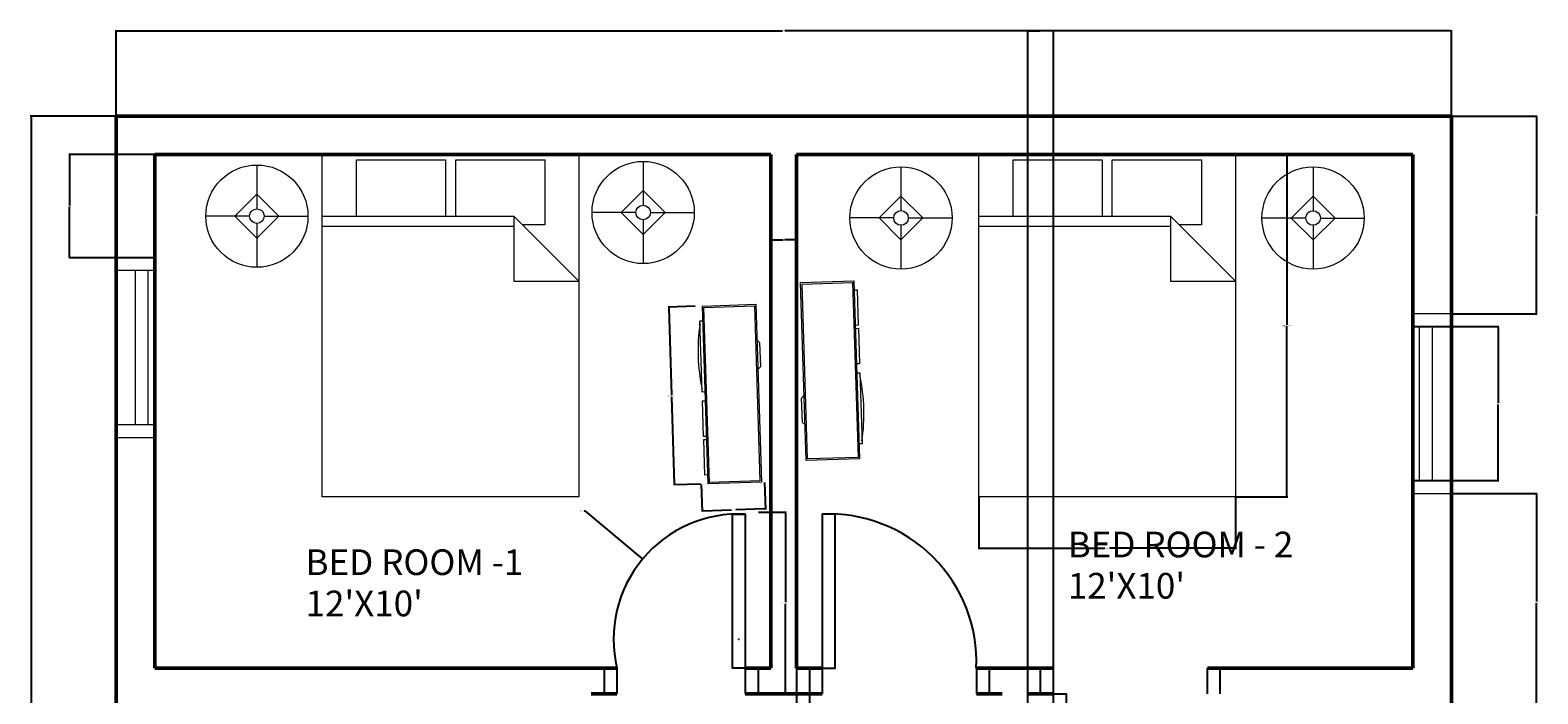
# Model space of a CAD drawing. Units: inches. Extents: x 2630 to 2982, y 643 to 1079.
# Tile 4 of 4: x 2630 to 2982, y 924 to 1079. Entities that reach past the tile are written whole.
import ezdxf

# ---------------------------------------------------------------- set-up
doc = ezdxf.new("R2010")
doc.units = ezdxf.units.IN
for name, color, linetype, lineweight in [('A-ANNO-DIMS', 2, 'Continuous', 18), ('A-AREA-IDEN', 7, 'Continuous', 25), ('A-DOOR', 3, 'Continuous', 25), ('A-FURN', 8, 'Continuous', 18), ('A-GLAZ', 4, 'Continuous', 18), ('A-WALL', 7, 'Continuous', 50)]:
    doc.layers.add(name, color=color, linetype=linetype, lineweight=lineweight)
doc.styles.get("Standard").update_dxf_attribs({"font": 'arial.ttf'})
doc.dimstyles.get("Standard").update_dxf_attribs({"dimtxt": 0.18, "dimasz": 0.18, "dimexe": 0.18, "dimexo": 0.0625, "dimgap": 0.09, "dimtad": 0, "dimtih": 1, "dimtoh": 1, "dimdec": 4, "dimzin": 0, "dimdsep": 46, "dimtxsty": 'Standard', "dimcen": 0.09, "dimadec": 0, "dimazin": 0, "dimtfac": 1, "dimtdec": 4, "dimtofl": 0, "dimtmove": 0, "dimatfit": 3, "dimfxl": 1, "dimtolj": 1, "dimtzin": 0, "dimarcsym": 0})

# ---------------------------------------------------------------- blocks, each defined once
blk = doc.blocks.new('Bed - Queen')
for p, q in [((0, -80.00003), (0, 0)), ((0, 0), (59.99999, 0)), ((59.99999, 0), (59.99999, -80.00003)), ((7.99999, -1.2), (28.79998, -1.2)), ((7.99999, -14.4), (7.99999, -1.2)), ((28.79998, -1.2), (28.79998, -14.4)), ((31.19999, -1.2), (51.99999, -1.2)), ((31.19999, -14.4), (31.19999, -1.2)), ((51.99999, -1.2), (51.99999, -16.4)), ((0, -14.4), (44.8, -14.4)), ((44.8, -16.8), (0, -16.8)), ((59.99999, -29.6), (44.8, -14.4)), ((44.8, -14.4), (44.8, -29.6)), ((51.99999, -16.4), (46.79936, -16.4)), ((44.8, -29.6), (59.99999, -29.6)), ((59.99999, -80.00003), (0, -80.00003))]:
    blk.add_line(p, q)
blk = doc.blocks.new('Lamp - Table')
for p, q in [((0, 7), (0, 1)), ((0, 3), (-3, 0)), ((3, 0), (0, 3)), ((-1, 0), (-7, 0)), ((-3, 0), (0, -3)), ((0, -3), (3, 0)), ((1, 0), (7, 0)), ((0, -1), (0, -7))]:
    blk.add_line(p, q)
for radius in [7, 1]:
    blk.add_circle((0, 0), radius)
blk = doc.blocks.new('Entertainment Center')
for p, q in [((-4, 0), (-5, -1)), ((4, 0), (-4, 0)), ((5, -1), (4, 0)), ((-17, -19), (-17, -1)), ((-17, -1), (43, -1)), ((-16.5, -18.5), (-16.5, -1.5)), ((-16.5, -1.5), (42.5, -1.5)), ((42.5, -1.5), (42.5, -18.5)), ((43, -1), (43, -19)), ((43, -19), (-17, -19)), ((42.5, -18.5), (-16.5, -18.5)), ((-12, -20), (-12, -19)), ((12, -20), (-12, -20)), ((12, -19), (12, -20)), ((15, -20), (15, -19)), ((27, -20), (15, -20)), ((27, -19), (27, -20)), ((28, -20), (28, -19)), ((40, -20), (28, -20)), ((40, -19), (40, -20))]:
    blk.add_line(p, q)
blk.add_arc((0, 40), 61, 259.6111, 280.3889)
blk = doc.blocks.new('DOOR-30IN-INT')
for p, q in [((0, 6), (0, 0)), ((3, 6), (3, 0)), ((33, 6), (33, 0)), ((36, 6), (36, 0))]:
    blk.add_line(p, q)
blk.add_lwpolyline([(33, 6), (30, 6), (30, 42), (33, 42)], close=True)
blk.add_arc((31.5, 12.75), 29.29, 87.0643, 193.3245)
blk = doc.blocks.new('DOOR-36IN-INT')
for p, q in [((0, 6), (0, 0)), ((3, 6), (3, 0)), ((39, 6), (39, 0)), ((42, 6), (42, 0))]:
    blk.add_line(p, q)
blk.add_lwpolyline([(3, 6), (6, 6), (6, 42), (3, 42)], close=True)
blk.add_arc((4.5, 7.5), 34.53, 357.5104, 92.4896)
blk = doc.blocks.new('WIN-36IN')
for p, q in [((9, 42), (0, 42)), ((9, 39), (0, 39)), ((4.5, 3), (4.5, 39)), ((7.5, 3), (7.5, 39)), ((0, 3), (9, 3)), ((0, 0), (9, 0))]:
    blk.add_line(p, q)
blk = doc.blocks.new('*D17')
at = {"layer": 'A-ANNO-DIMS', "color": 0, "lineweight": -2, "transparency": 16777216}
for p, q in [((2911.41, 1049.87), (2923.53, 1049.87)), ((2923.35, 1049.69), (2923.35, 1010.06)), ((2923.35, 970.05), (2923.35, 1009.68)), ((2911.41, 969.87), (2923.53, 969.87))]:
    blk.add_line(p, q, dxfattribs=at)
at = {"layer": 'A-ANNO-DIMS', "color": 0, "transparency": 16777216}
for points in [[(2923.32, 1049.69), (2923.38, 1049.69), (2923.35, 1049.87)], [(2923.32, 970.05), (2923.38, 970.05), (2923.35, 969.87)]]:
    blk.add_solid(points, dxfattribs=at)
at = {"layer": 'Defpoints', "color": 0, "transparency": 16777216}
for p in [(2911.35, 1049.87), (2923.35, 1049.87), (2911.35, 969.87)]:
    blk.add_point(p, dxfattribs=at)
at = {"layer": 'A-ANNO-DIMS', "color": 0, "transparency": 16777216, "insert": (2923.35, 1009.87), "char_height": 0.18, "attachment_point": 5}
blk.add_mtext('\\A1;QUEEN BED 80 TYP.', dxfattribs=at)
blk = doc.blocks.new('*D18')
at = {"layer": 'A-ANNO-DIMS', "color": 0, "lineweight": -2, "transparency": 16777216}
for p, q in [((2851.35, 969.8), (2851.35, 957.69)), ((2911.35, 969.8), (2911.35, 957.69)), ((2851.53, 957.87), (2880.82, 957.87)), ((2911.17, 957.87), (2881.87, 957.87))]:
    blk.add_line(p, q, dxfattribs=at)
at = {"layer": 'A-ANNO-DIMS', "color": 0, "transparency": 16777216}
for points in [[(2851.53, 957.9), (2851.53, 957.84), (2851.35, 957.87)], [(2911.17, 957.9), (2911.17, 957.84), (2911.35, 957.87)]]:
    blk.add_solid(points, dxfattribs=at)
at = {"layer": 'Defpoints', "color": 0, "transparency": 16777216}
for p in [(2851.35, 969.87), (2911.35, 969.87), (2911.35, 957.87)]:
    blk.add_point(p, dxfattribs=at)
at = {"layer": 'A-ANNO-DIMS', "color": 0, "transparency": 16777216, "insert": (2881.35, 957.87), "char_height": 0.18, "attachment_point": 5}
blk.add_mtext('\\A1;60 TYP.', dxfattribs=at)
blk = doc.blocks.new('*D23')
at = {"layer": 'A-ANNO-DIMS', "color": 0, "lineweight": -2, "transparency": 16777216}
for p, q in [((2785.08, 1014.44), (2778.72, 1014.24)), ((2778.91, 1014.06), (2779.56, 993.64)), ((2780.23, 972.86), (2779.58, 993.28)), ((2786.41, 972.88), (2780.06, 972.67))]:
    blk.add_line(p, q, dxfattribs=at)
at = {"layer": 'A-ANNO-DIMS', "color": 0, "transparency": 16777216}
for points in [[(2778.94, 1014.06), (2778.88, 1014.06), (2778.9, 1014.24)], [(2780.26, 972.86), (2780.2, 972.86), (2780.24, 972.68)]]:
    blk.add_solid(points, dxfattribs=at)
at = {"layer": 'Defpoints', "color": 0, "transparency": 16777216}
for p in [(2785.14, 1014.44), (2780.24, 972.68), (2786.47, 972.88)]:
    blk.add_point(p, dxfattribs=at)
at = {"layer": 'A-ANNO-DIMS', "color": 0, "transparency": 16777216, "insert": (2779.57, 993.46), "char_height": 0.18, "attachment_point": 5}
blk.add_mtext('\\A1;MEDIA UNIT 42 TYP.', dxfattribs=at)
blk = doc.blocks.new('*D24')
at = {"layer": 'A-ANNO-DIMS', "color": 0, "lineweight": -2, "transparency": 16777216}
for p, q in [((2786.47, 972.82), (2786.68, 966.47)), ((2801.25, 973.29), (2801.46, 966.94)), ((2786.85, 966.65), (2793.54, 966.87)), ((2801.27, 967.11), (2794.58, 966.9))]:
    blk.add_line(p, q, dxfattribs=at)
at = {"layer": 'A-ANNO-DIMS', "color": 0, "transparency": 16777216}
for points in [[(2786.85, 966.68), (2786.85, 966.62), (2786.67, 966.65)], [(2801.27, 967.14), (2801.27, 967.08), (2801.45, 967.12)]]:
    blk.add_solid(points, dxfattribs=at)
at = {"layer": 'Defpoints', "color": 0, "transparency": 16777216}
for p in [(2786.47, 972.88), (2801.25, 973.35), (2801.45, 967.12)]:
    blk.add_point(p, dxfattribs=at)
at = {"layer": 'A-ANNO-DIMS', "color": 0, "transparency": 16777216, "insert": (2794.06, 966.88), "char_height": 0.18, "attachment_point": 5}
blk.add_mtext('\\A1;15 TYP.', dxfattribs=at)
blk = doc.blocks.new('*D25')
at = {"layer": 'A-ANNO-DIMS', "color": 0, "lineweight": -2, "transparency": 16777216}
for p, q in [((2799.83, 966.34), (2806.32, 966.34)), ((2806.14, 966.16), (2806.14, 945.29)), ((2806.14, 924.05), (2806.14, 944.92)), ((2799.83, 923.87), (2806.32, 923.87))]:
    blk.add_line(p, q, dxfattribs=at)
at = {"layer": 'A-ANNO-DIMS', "color": 0, "transparency": 16777216}
for points in [[(2806.11, 966.16), (2806.17, 966.16), (2806.14, 966.34)], [(2806.11, 924.05), (2806.17, 924.05), (2806.14, 923.87)]]:
    blk.add_solid(points, dxfattribs=at)
at = {"layer": 'Defpoints', "color": 0, "transparency": 16777216}
for p in [(2799.77, 966.34), (2806.14, 966.34), (2799.77, 923.87)]:
    blk.add_point(p, dxfattribs=at)
at = {"layer": 'A-ANNO-DIMS', "color": 0, "transparency": 16777216, "insert": (2806.14, 945.1), "char_height": 0.18, "attachment_point": 5}
blk.add_mtext('\\A1;DOOR D2 42 TYP.', dxfattribs=at)
blk = doc.blocks.new('*D37')
at = {"layer": 'A-ANNO-DIMS', "color": 0, "lineweight": -2, "transparency": 16777216}
for p, q in [((2649.77, 1058.93), (2649.77, 1078.96)), ((2649.95, 1078.78), (2805.48, 1078.78)), ((2961.59, 1078.78), (2806.05, 1078.78)), ((2961.77, 1058.93), (2961.77, 1078.96))]:
    blk.add_line(p, q, dxfattribs=at)
at = {"layer": 'A-ANNO-DIMS', "color": 0, "transparency": 16777216}
for points in [[(2649.95, 1078.81), (2649.95, 1078.75), (2649.77, 1078.78)], [(2961.59, 1078.81), (2961.59, 1078.75), (2961.77, 1078.78)]]:
    blk.add_solid(points, dxfattribs=at)
at = {"layer": 'Defpoints', "color": 0, "transparency": 16777216}
for p in [(2961.77, 1078.78), (2649.77, 1058.87), (2961.77, 1058.87)]:
    blk.add_point(p, dxfattribs=at)
at = {"layer": 'A-ANNO-DIMS', "color": 0, "transparency": 16777216, "insert": (2805.77, 1078.78), "char_height": 0.18, "attachment_point": 5}
blk.add_mtext('\\A1;312', dxfattribs=at)
blk = doc.blocks.new('*D38')
at = {"layer": 'A-ANNO-DIMS', "color": 0, "lineweight": -2, "transparency": 16777216}
for p, q in [((2649.7, 1058.87), (2629.68, 1058.87)), ((2629.86, 1058.69), (2629.86, 861.05)), ((2629.86, 663.05), (2629.86, 860.68)), ((2649.7, 662.87), (2629.68, 662.87))]:
    blk.add_line(p, q, dxfattribs=at)
at = {"layer": 'A-ANNO-DIMS', "color": 0, "transparency": 16777216}
for points in [[(2629.83, 1058.69), (2629.89, 1058.69), (2629.86, 1058.87)], [(2629.83, 663.05), (2629.89, 663.05), (2629.86, 662.87)]]:
    blk.add_solid(points, dxfattribs=at)
at = {"layer": 'Defpoints', "color": 0, "transparency": 16777216}
for p in [(2629.86, 1058.87), (2649.77, 1058.87), (2649.77, 662.87)]:
    blk.add_point(p, dxfattribs=at)
at = {"layer": 'A-ANNO-DIMS', "color": 0, "transparency": 16777216, "insert": (2629.86, 860.87), "char_height": 0.18, "attachment_point": 5}
blk.add_mtext('\\A1;396', dxfattribs=at)
blk = doc.blocks.new('*D40')
at = {"layer": 'A-ANNO-DIMS', "color": 0, "lineweight": -2, "transparency": 16777216}
for p, q in [((2802.77, 1049.8), (2802.77, 1029.78)), ((2808.77, 1049.8), (2808.77, 1029.78)), ((2802.95, 1029.96), (2805.62, 1029.96)), ((2808.59, 1029.96), (2805.92, 1029.96))]:
    blk.add_line(p, q, dxfattribs=at)
at = {"layer": 'A-ANNO-DIMS', "color": 0, "transparency": 16777216}
for points in [[(2802.95, 1029.99), (2802.95, 1029.93), (2802.77, 1029.96)], [(2808.59, 1029.99), (2808.59, 1029.93), (2808.77, 1029.96)]]:
    blk.add_solid(points, dxfattribs=at)
at = {"layer": 'Defpoints', "color": 0, "transparency": 16777216}
for p in [(2802.77, 1049.87), (2808.77, 1049.87), (2802.77, 1029.96)]:
    blk.add_point(p, dxfattribs=at)
at = {"layer": 'A-ANNO-DIMS', "color": 0, "transparency": 16777216, "insert": (2805.77, 1029.96), "char_height": 0.18, "attachment_point": 5}
blk.add_mtext('\\A1;6', dxfattribs=at)
blk = doc.blocks.new('*D41')
at = {"layer": 'A-ANNO-DIMS', "color": 0, "lineweight": -2, "transparency": 16777216}
for p, q in [((2658.7, 1049.87), (2638.68, 1049.87)), ((2638.86, 1049.69), (2638.86, 1038)), ((2638.86, 1025.95), (2638.86, 1037.64)), ((2658.7, 1025.77), (2638.68, 1025.77))]:
    blk.add_line(p, q, dxfattribs=at)
at = {"layer": 'A-ANNO-DIMS', "color": 0, "transparency": 16777216}
for points in [[(2638.83, 1049.69), (2638.89, 1049.69), (2638.86, 1049.87)], [(2638.83, 1025.95), (2638.89, 1025.95), (2638.86, 1025.77)]]:
    blk.add_solid(points, dxfattribs=at)
at = {"layer": 'Defpoints', "color": 0, "transparency": 16777216}
for p in [(2638.86, 1049.87), (2658.77, 1049.87), (2658.77, 1025.77)]:
    blk.add_point(p, dxfattribs=at)
at = {"layer": 'A-ANNO-DIMS', "color": 0, "transparency": 16777216, "insert": (2638.86, 1037.82), "char_height": 0.18, "attachment_point": 5}
blk.add_mtext('\\A1;24.093', dxfattribs=at)
blk = doc.blocks.new('*D45')
at = {"layer": 'A-ANNO-DIMS', "color": 0, "lineweight": -2, "transparency": 16777216}
for p, q in [((2961.83, 1058.87), (2981.86, 1058.87)), ((2981.68, 1058.69), (2981.68, 1035.96)), ((2981.68, 1012.87), (2981.68, 1035.6)), ((2961.83, 1012.69), (2981.86, 1012.69))]:
    blk.add_line(p, q, dxfattribs=at)
at = {"layer": 'A-ANNO-DIMS', "color": 0, "transparency": 16777216}
for points in [[(2981.65, 1058.69), (2981.71, 1058.69), (2981.68, 1058.87)], [(2981.65, 1012.87), (2981.71, 1012.87), (2981.68, 1012.69)]]:
    blk.add_solid(points, dxfattribs=at)
at = {"layer": 'Defpoints', "color": 0, "transparency": 16777216}
for p in [(2961.77, 1058.87), (2961.77, 1012.69), (2981.68, 1012.69)]:
    blk.add_point(p, dxfattribs=at)
at = {"layer": 'A-ANNO-DIMS', "color": 0, "transparency": 16777216, "insert": (2981.68, 1035.78), "char_height": 0.18, "attachment_point": 5}
blk.add_mtext('\\A1;46.18', dxfattribs=at)
blk = doc.blocks.new('*D46')
at = {"layer": 'A-ANNO-DIMS', "color": 0, "lineweight": -2, "transparency": 16777216}
for p, q in [((2961.83, 970.69), (2981.86, 970.69)), ((2981.68, 970.51), (2981.68, 945.45)), ((2981.68, 920.02), (2981.68, 945.08)), ((2961.83, 919.84), (2981.86, 919.84))]:
    blk.add_line(p, q, dxfattribs=at)
at = {"layer": 'A-ANNO-DIMS', "color": 0, "transparency": 16777216}
for points in [[(2981.65, 970.51), (2981.71, 970.51), (2981.68, 970.69)], [(2981.65, 920.02), (2981.71, 920.02), (2981.68, 919.84)]]:
    blk.add_solid(points, dxfattribs=at)
at = {"layer": 'Defpoints', "color": 0, "transparency": 16777216}
for p in [(2961.77, 970.69), (2981.68, 970.69), (2961.77, 919.84)]:
    blk.add_point(p, dxfattribs=at)
at = {"layer": 'A-ANNO-DIMS', "color": 0, "transparency": 16777216, "insert": (2981.68, 945.27), "char_height": 0.18, "attachment_point": 5}
blk.add_mtext('\\A1;50.85', dxfattribs=at)
blk = doc.blocks.new('*D58')
at = {"layer": 'A-ANNO-DIMS', "color": 0, "lineweight": -2, "transparency": 16777216}
for p, q in [((2862.77, 767.93), (2862.77, 1078.96)), ((2862.95, 1078.78), (2865.62, 1078.78)), ((2868.59, 1078.78), (2865.92, 1078.78)), ((2868.77, 767.93), (2868.77, 1078.96))]:
    blk.add_line(p, q, dxfattribs=at)
at = {"layer": 'A-ANNO-DIMS', "color": 0, "transparency": 16777216}
for points in [[(2862.95, 1078.81), (2862.95, 1078.75), (2862.77, 1078.78)], [(2868.59, 1078.81), (2868.59, 1078.75), (2868.77, 1078.78)]]:
    blk.add_solid(points, dxfattribs=at)
at = {"layer": 'Defpoints', "color": 0, "transparency": 16777216}
for p in [(2868.77, 1078.78), (2862.77, 767.87), (2868.77, 767.87)]:
    blk.add_point(p, dxfattribs=at)
at = {"layer": 'A-ANNO-DIMS', "color": 0, "transparency": 16777216, "insert": (2865.77, 1078.78), "char_height": 0.18, "attachment_point": 5}
blk.add_mtext('\\A1;6', dxfattribs=at)
blk = doc.blocks.new('*D59')
at = {"layer": 'A-ANNO-DIMS', "color": 0, "lineweight": -2, "transparency": 16777216}
for p, q in [((2808.77, 929.8), (2808.77, 642.78)), ((2811.77, 929.8), (2811.77, 642.78)), ((2808.95, 642.96), (2810.12, 642.96)), ((2811.59, 642.96), (2810.42, 642.96))]:
    blk.add_line(p, q, dxfattribs=at)
at = {"layer": 'A-ANNO-DIMS', "color": 0, "transparency": 16777216}
for points in [[(2808.95, 642.99), (2808.95, 642.93), (2808.77, 642.96)], [(2811.59, 642.99), (2811.59, 642.93), (2811.77, 642.96)]]:
    blk.add_solid(points, dxfattribs=at)
at = {"layer": 'Defpoints', "color": 0, "transparency": 16777216}
for p in [(2808.77, 929.87), (2811.77, 929.87), (2811.77, 642.96)]:
    blk.add_point(p, dxfattribs=at)
at = {"layer": 'A-ANNO-DIMS', "color": 0, "transparency": 16777216, "insert": (2810.27, 642.96), "char_height": 0.18, "attachment_point": 5}
blk.add_mtext('\\A1;3', dxfattribs=at)
blk = doc.blocks.new('*D66')
at = {"layer": 'A-ANNO-DIMS', "color": 0, "lineweight": -2, "transparency": 16777216}
for p, q in [((2952.83, 1009.69), (2972.86, 1009.69)), ((2972.68, 1009.51), (2972.68, 991.87)), ((2972.68, 973.87), (2972.68, 991.51)), ((2952.83, 973.69), (2972.86, 973.69))]:
    blk.add_line(p, q, dxfattribs=at)
at = {"layer": 'A-ANNO-DIMS', "color": 0, "transparency": 16777216}
for points in [[(2972.65, 1009.51), (2972.71, 1009.51), (2972.68, 1009.69)], [(2972.65, 973.87), (2972.71, 973.87), (2972.68, 973.69)]]:
    blk.add_solid(points, dxfattribs=at)
at = {"layer": 'Defpoints', "color": 0, "transparency": 16777216}
for p in [(2952.77, 1009.69), (2952.77, 973.69), (2972.68, 973.69)]:
    blk.add_point(p, dxfattribs=at)
at = {"layer": 'A-ANNO-DIMS', "color": 0, "transparency": 16777216, "insert": (2972.68, 991.69), "char_height": 0.18, "attachment_point": 5}
blk.add_mtext('\\A1;36', dxfattribs=at)
blk = doc.blocks.new('*D68')
at = {"layer": 'A-ANNO-DIMS', "color": 0, "lineweight": -2, "transparency": 16777216}
for p, q in [((2759.09, 966.62), (2759.27, 966.62)), ((2759.27, 966.62), (2772.63, 955.48)), ((2795.18, 936.62), (2795.36, 936.62)), ((2795.27, 936.53), (2795.27, 936.71))]:
    blk.add_line(p, q, dxfattribs=at)
at = {"layer": 'A-ANNO-DIMS', "color": 0, "transparency": 16777216}
blk.add_solid([(2772.65, 955.51), (2772.61, 955.46), (2772.77, 955.37)], dxfattribs=at)
at = {"layer": 'Defpoints', "color": 0, "transparency": 16777216}
for p in [(2772.77, 955.37), (2795.27, 936.62)]:
    blk.add_point(p, dxfattribs=at)
at = {"layer": 'A-ANNO-DIMS', "color": 0, "transparency": 16777216, "insert": (2758.61, 966.62), "char_height": 0.18, "attachment_point": 5}
blk.add_mtext('\\A1;R29.29', dxfattribs=at)

msp = doc.modelspace()

# ---------------------------------------------------------------- linework, layer by layer
at = {"layer": 'A-DOOR'}
for p, q in [((2865.7671, 923.8666), (2865.7671, 929.8666)), ((2868.7671, 923.8666), (2868.7671, 929.8666)), ((2904.7671, 923.8666), (2904.7671, 929.8666)), ((2907.7671, 923.8666), (2907.7671, 929.8666))]:
    msp.add_line(p, q, dxfattribs=at)
msp.add_lwpolyline([(2868.7671, 923.8666), (2871.7671, 923.8666), (2871.7671, 887.8666), (2868.7671, 887.8666)], close=True, dxfattribs=at)
at = {"layer": 'A-WALL'}
for p, q in [((2658.7671, 1049.8666), (2658.7671, 929.8666)), ((2802.7671, 1049.8666), (2658.7671, 1049.8666)), ((2802.7671, 1049.8666), (2802.7671, 929.8666)), ((2952.7671, 1049.8666), (2808.7671, 1049.8666)), ((2808.7671, 1049.8666), (2808.7671, 929.8666)), ((2952.7671, 929.8666), (2952.7671, 1049.8666)), ((2766.7671, 929.8666), (2658.7671, 929.8666)), ((2802.7671, 929.8666), (2796.7671, 929.8666)), ((2814.7671, 929.8666), (2808.7671, 929.8666)), ((2868.7671, 929.8666), (2850.7671, 929.8666)), ((2952.7671, 929.8666), (2904.7671, 929.8666)), ((2766.7671, 923.8666), (2760.7671, 923.8666)), ((2814.7671, 923.8666), (2796.7671, 923.8666)), ((2856.7671, 923.8666), (2850.7671, 923.8666)), ((2868.7671, 923.8666), (2862.7671, 923.8666))]:
    msp.add_line(p, q, dxfattribs=at)
msp.add_lwpolyline([(2850.7671, 662.8666), (2961.7671, 662.8666), (2961.7671, 1058.8666), (2649.7671, 1058.8666), (2649.7671, 662.8666), (2814.7671, 662.8666)], dxfattribs=at)

# ---------------------------------------------------------------- block references
at = {"layer": 'A-DOOR'}
for name, p in [('DOOR-30IN-INT', (2763.767, 923.867)), ('DOOR-36IN-INT', (2811.767, 923.867))]:
    msp.add_blockref(name, p, dxfattribs=at)
at = {"layer": 'A-FURN', "xscale": 1.706595897520738, "yscale": 1.706595897520738, "zscale": 1.706595897520738}
for p in [(2682.6314, 1035.4951), (2772.9035, 1036.3461), (2833.1558, 1035.0697), (2929.4613, 1035.0588)]:
    msp.add_blockref('Lamp - Table', p, dxfattribs=at)
at = {"layer": 'A-FURN'}
for p in [(2697.8913, 1049.8666), (2851.3458, 1049.8666)]:
    msp.add_blockref('Bed - Queen', p, dxfattribs=at)
at = {"layer": 'A-FURN', "xscale": 0.6930832416861975, "yscale": 0.6930832416861975, "zscale": 0.6930832416861975}
for p, rotation in [((2809.9377, 990.1498), 91.83802292869142), ((2800.2946, 1003.1413), 271.8380229286914)]:
    msp.add_blockref('Entertainment Center', p, dxfattribs=dict(at, rotation=rotation))
at = {"layer": 'A-GLAZ'}
msp.add_blockref('WIN-36IN', (2649.767, 983.774), dxfattribs=at)
at = {"layer": 'A-GLAZ', "rotation": 180}
msp.add_blockref('WIN-36IN', (2961.7672, 1012.6884), dxfattribs=at)

# ---------------------------------------------------------------- texts
at = {"layer": 'A-AREA-IDEN'}
for s, p in [('BED ROOM - 2', (2872.1286, 955.7588)), ('BED ROOM -1', (2694.0093, 951.6277)), ("12'X10'", (2872.1286, 946.1203)), ("12'X10'", (2694.0093, 941.9892))]:
    msp.add_text(s, height=6, dxfattribs=at).set_placement(p)

# ---------------------------------------------------------------- dimensions: what is measured, and where the dimension line sits
at = {"layer": 'A-ANNO-DIMS'}
for base, p1, p2, picture, middle in [((2961.7671, 1078.7766), (2649.7671, 1058.8666), (2961.7671, 1058.8666), '*D37', (2805.7671, 1078.7766)), ((2868.7671, 1078.7766), (2862.7671, 767.8666), (2868.7671, 767.8666), '*D58', (2865.7671, 1078.7766)), ((2811.7671, 642.9566), (2808.7671, 929.8666), (2811.7671, 929.8666), '*D59', (2810.2671, 642.9566))]:
    dim = msp.add_linear_dim(base=base, p1=p1, p2=p2, dimstyle='Standard', override={"dimdec": 0, "dimlfac": 1, "dimrnd": 0, "dimzin": 0, "dimdsep": 46, "dimlunit": 2}, dxfattribs=at)
    dim.commit()
    dim.dimension.update_dxf_attribs({"geometry": picture, "text_midpoint": middle})
for base, p1, p2, angle, override, picture, middle in [((2629.8571, 1058.8666), (2649.7671, 662.8666), (2649.7671, 1058.8666), 90, {"dimdec": 0, "dimlfac": 1, "dimrnd": 0, "dimzin": 0, "dimdsep": 46, "dimlunit": 2}, '*D38', (2629.8571, 860.8666)), ((2981.6771, 1012.6885), (2961.7671, 1058.8666), (2961.7671, 1012.6885), 90, {"dimdec": 2, "dimlfac": 1, "dimrnd": 0, "dimzin": 0, "dimdsep": 46, "dimlunit": 2}, '*D45', (2981.6771, 1035.7775)), ((2638.8571, 1049.8666), (2658.7671, 1025.7739), (2658.7671, 1049.8666), 90, {"dimdec": 3, "dimlfac": 1, "dimrnd": 0, "dimzin": 0, "dimdsep": 46, "dimlunit": 2}, '*D41', (2638.8571, 1037.8203)), ((2802.7671, 1029.9566), (2808.7671, 1049.8666), (2802.7671, 1049.8666), 180, {"dimdec": 0, "dimlfac": 1, "dimrnd": 0, "dimzin": 0, "dimdsep": 46, "dimlunit": 2}, '*D40', (2805.7671, 1029.9566)), ((2972.6771, 973.6885), (2952.7671, 1009.6885), (2952.7671, 973.6885), 270, {"dimdec": 0, "dimlfac": 1, "dimrnd": 0, "dimzin": 0, "dimdsep": 46, "dimlunit": 2}, '*D66', (2972.6771, 991.6885)), ((2981.6771, 970.6885), (2961.7671, 919.8429), (2961.7671, 970.6885), 90, {"dimdec": 2, "dimlfac": 1, "dimrnd": 0, "dimzin": 0, "dimdsep": 46, "dimlunit": 2}, '*D46', (2981.6771, 945.2657))]:
    dim = msp.add_linear_dim(base=base, p1=p1, p2=p2, angle=angle, dimstyle='Standard', override=override, dxfattribs=at)
    dim.commit()
    dim.dimension.update_dxf_attribs({"geometry": picture, "text_midpoint": middle})
for base, p1, p2, angle, text, picture, middle in [((2923.3458, 1049.8666), (2911.3458, 969.8666), (2911.3458, 1049.8666), 90, 'QUEEN BED <> TYP.', '*D17', (2923.3458, 1009.8666)), ((2780.2377, 972.6798), (2785.1385, 1014.4434), (2786.4723, 972.8798), 271.838023, 'MEDIA UNIT <> TYP.', '*D23', (2779.5708, 993.4616)), ((2801.4505, 967.1195), (2786.4723, 972.8798), (2801.2504, 973.3541), 1.838023, '<> TYP.', '*D24', (2794.0614, 966.8824)), ((2806.1379, 966.3388), (2799.7671, 923.8666), (2799.7671, 966.3388), 90, 'DOOR D2 <> TYP.', '*D25', (2806.1379, 945.1027))]:
    dim = msp.add_linear_dim(base=base, p1=p1, p2=p2, angle=angle, text=text, dimstyle='Standard', override={"dimdec": 0, "dimlfac": 1, "dimrnd": 0, "dimzin": 0, "dimdsep": 46, "dimlunit": 2}, dxfattribs=at)
    dim.commit()
    dim.dimension.update_dxf_attribs({"geometry": picture, "text_midpoint": middle})
dim = msp.add_linear_dim(base=(2911.3458, 957.8666), p1=(2851.3458, 969.8666), p2=(2911.3458, 969.8666), text='<> TYP.', dimstyle='Standard', override={"dimdec": 0, "dimlfac": 1, "dimrnd": 0, "dimzin": 0, "dimdsep": 46, "dimlunit": 2}, dxfattribs=at)
dim.commit()
dim.dimension.update_dxf_attribs({"geometry": '*D18', "text_midpoint": (2881.3458, 957.8666)})
dim = msp.add_radius_dim(center=(2795.2671, 936.6166), mpoint=(2772.7672, 955.3668), dimstyle='Standard', override={"dimdec": 2, "dimlfac": 1, "dimrnd": 0, "dimzin": 0, "dimdsep": 46, "dimlunit": 2}, dxfattribs=at)
dim.commit()
dim.dimension.update_dxf_attribs({"geometry": '*D68', "text_midpoint": (2758.6073, 966.6169), "dimtype": 164})

doc.saveas('drawing.dxf')
